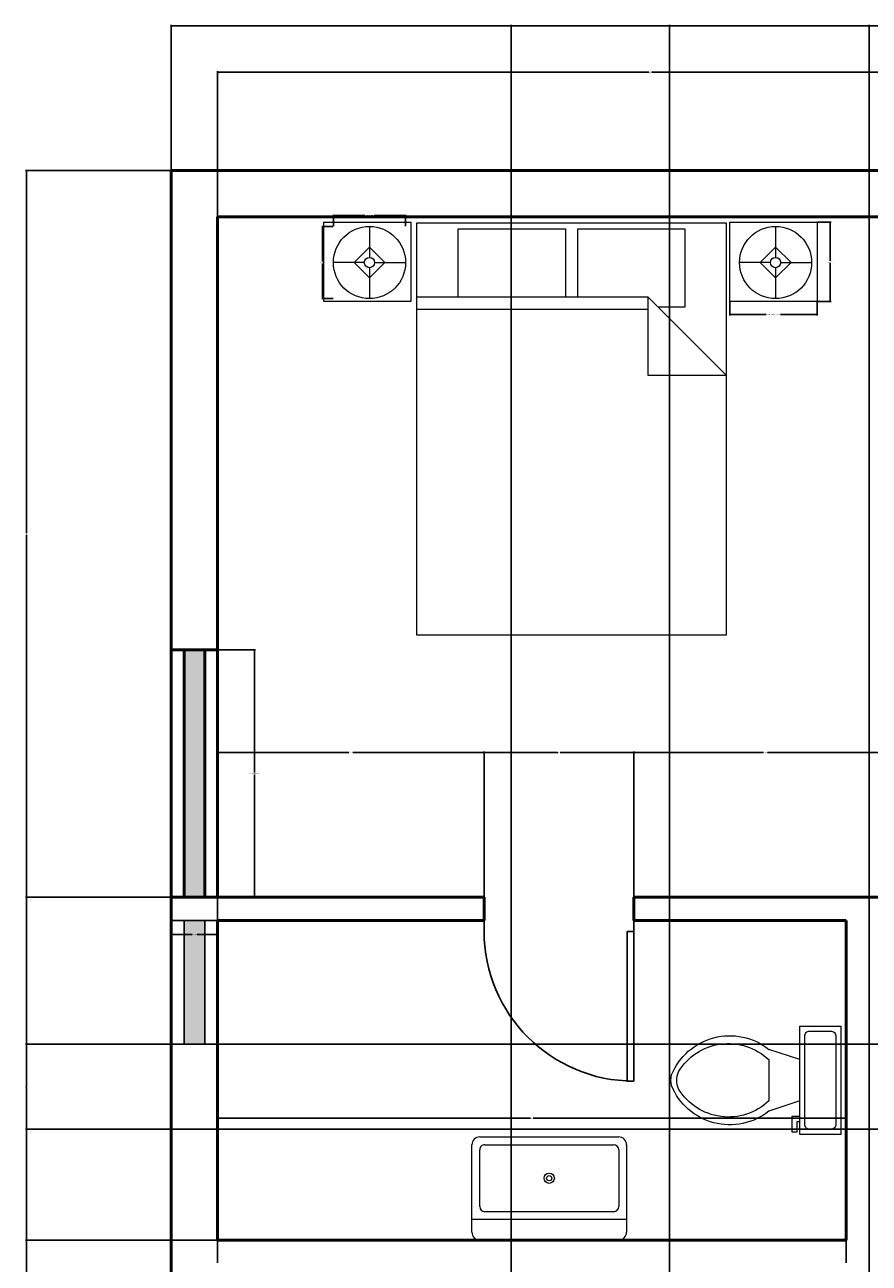
# Model space of a CAD drawing. Units: inches. Extents: x 1974 to 2406, y 1583 to 2170.
# Tile 4 of 6: x 1974 to 2138, y 1930 to 2170. Entities that reach past the tile are written whole.
import ezdxf

# ---------------------------------------------------------------- set-up
doc = ezdxf.new("R2010")
doc.units = ezdxf.units.IN
for name, color, linetype, lineweight in [('A-ANNO-DIMS', 2, 'Continuous', 18), ('A-FLOR-FIXT', 3, 'Continuous', 18), ('A-FURN', 3, 'Continuous', 18), ('A-GLAZ', 4, 'Continuous', 25), ('door', 60, 'Continuous', 25), ('wall', 240, 'Continuous', 50)]:
    doc.layers.add(name, color=color, linetype=linetype, lineweight=lineweight)
doc.styles.get("Standard").update_dxf_attribs({"font": 'arial.ttf'})
doc.dimstyles.get("Standard").update_dxf_attribs({"dimtxt": 0.18, "dimasz": 0.18, "dimexe": 0.18, "dimexo": 0.0625, "dimgap": 0.09, "dimtad": 0, "dimtih": 1, "dimtoh": 1, "dimdec": 4, "dimzin": 0, "dimdsep": 46, "dimtxsty": 'Standard', "dimcen": 0.09, "dimadec": 0, "dimazin": 0, "dimtfac": 1, "dimtdec": 4, "dimtofl": 0, "dimtmove": 0, "dimatfit": 3, "dimfxl": 1, "dimtolj": 1, "dimtzin": 0, "dimarcsym": 0})

# ---------------------------------------------------------------- blocks, each defined once
blk = doc.blocks.new('*U2')
for p, q in [((0, 0), (0, -6)), ((40, 0), (40, -6))]:
    blk.add_line(p, q)
blk.add_lwpolyline([(0, 0), (0, 40), (1.75, 40), (1.75, 0)], close=True)
blk.add_arc((0, 0), 40, 0, 90)
blk = doc.blocks.new('b')
at = {"layer": 'wall'}
h = blk.add_hatch(color=256, dxfattribs=at)
h.dxf.hatch_style = 1
h.paths.add_polyline_path([(6.5, 0), (2.5, 0), (2.5, -48), (6.5, -48)])
for p, q in [((2.5, 0), (2.5, -48)), ((6.5, 0), (6.5, -48))]:
    blk.add_line(p, q, dxfattribs=at)
blk.add_lwpolyline([(0, -48), (9, -48), (9, 0), (0, 0)], close=True, dxfattribs=at)
blk = doc.blocks.new('*U7')
for p, q in [((9.5, -6), (9.5, -2)), ((-10, -8.5), (-8, -8.5)), ((-10, -9.5), (-10, -8.5)), ((-7, -9.5), (-10, -9.5)), ((-8, -8.5), (-8, -8)), ((-7, -8), (-7, -9.5)), ((-4, -8), (-6, -14)), ((4, -8), (6, -14)), ((4, -14), (-4, -14))]:
    blk.add_line(p, q)
blk.add_lwpolyline([(10.5, -8), (10.5, 0), (-10.5, 0), (-10.5, -8)], close=True)
for points in [[(-9.5, -2), (-9.5, -6)], [(8.5, -1), (-8.5, -1)], [(-8.5, -7), (8.5, -7)]]:
    blk.add_lwpolyline(points)
for centre, radius, start, end in [((-8.62, -1.88), 0.884, 81.8699, 188.1301), ((8.62, -1.88), 0.884, 351.8699, 98.1301), ((-8.62, -6.12), 0.884, 171.8699, 278.1301), ((8.62, -6.12), 0.884, 261.8699, 8.1301), ((3.52, -21.58), 12.17, 141.4691, 247.9714), ((4.2, -21.82), 11.33, 136.3677, 238.9468), ((-3.52, -21.58), 12.17, 292.0284, 38.5307), ((-4.2, -21.82), 11.33, 301.053, 43.6321), ((0, -27.88), 4, 245.7318, 294.2682), ((0, -29), 4, 254.8605, 285.1395)]:
    blk.add_arc(centre, radius, start, end)
blk = doc.blocks.new('Sink-single - 30 in top')
blk.add_line((-15, -3.999996), (15, -3.999996))
for points in [[(-13.5, 0), (13.5, 0)], [(-15, -18.499996), (-15, -1.5)], [(15, -1.5), (15, -18.499996)], [(-13.5, -17.499996), (-13.5, -6.499996)], [(-12.5, -5.499996), (12.5, -5.499996)], [(13.5, -6.499996), (13.5, -17.499996)], [(12.5, -18.499996), (-12.5, -18.499996)], [(13.5, -19.999996), (-13.5, -19.999996)]]:
    blk.add_lwpolyline(points)
for radius in [1, 0.5]:
    blk.add_circle((0, -11.999996), radius)
for centre, radius, start, end in [((-13.5, -1.5), 1.5, 90, 180), ((13.5, -1.5), 1.5, 0, 90), ((-12.5, -6.499996), 1, 90, 180), ((12.5, -6.499996), 1, 0, 90), ((-13.5, -18.499996), 1.5, 180, 270), ((-12.5, -17.499996), 1, 180, 270), ((12.5, -17.499996), 1, 270, 0), ((13.5, -18.499996), 1.5, 270, 0)]:
    blk.add_arc(centre, radius, start, end)
blk = doc.blocks.new('Bed - Queen')
for p, q in [((0, -80.00003), (0, 0)), ((0, 0), (59.99999, 0)), ((59.99999, 0), (59.99999, -80.00003)), ((7.99999, -1.2), (28.79998, -1.2)), ((7.99999, -14.4), (7.99999, -1.2)), ((28.79998, -1.2), (28.79998, -14.4)), ((31.19999, -1.2), (51.99999, -1.2)), ((31.19999, -14.4), (31.19999, -1.2)), ((51.99999, -1.2), (51.99999, -16.4)), ((0, -14.4), (44.8, -14.4)), ((59.99999, -29.6), (44.8, -14.4)), ((44.8, -14.4), (44.8, -29.6)), ((44.8, -16.8), (0, -16.8)), ((51.99999, -16.4), (46.79936, -16.4)), ((44.8, -29.6), (59.99999, -29.6)), ((59.99999, -80.00003), (0, -80.00003))]:
    blk.add_line(p, q)
blk = doc.blocks.new('Lamp - Table')
for p, q in [((0, 7), (0, 1)), ((0, 3), (-3, 0)), ((3, 0), (0, 3)), ((-1, 0), (-7, 0)), ((-3, 0), (0, -3)), ((0, -3), (3, 0)), ((1, 0), (7, 0)), ((0, -1), (0, -7))]:
    blk.add_line(p, q)
for radius in [7, 1]:
    blk.add_circle((0, 0), radius)
blk = doc.blocks.new('WINDOW-24IN')
h = blk.add_hatch(color=256)
h.dxf.hatch_style = 1
h.paths.add_polyline_path([(6.5, 24), (2.5, 24), (2.5, 0), (6.5, 0)])
for p, q in [((2.5, 24), (2.5, 0)), ((6.5, 24), (6.5, 0))]:
    blk.add_line(p, q)
blk.add_lwpolyline([(0, 0), (0, 24), (9, 24), (9, 0)], close=True)
blk = doc.blocks.new('TABLE-NIGHTSTAND')
blk.add_lwpolyline([(0, 15.39), (16.93, 15.39), (16.93, 0), (0, 0)], close=True)
blk = doc.blocks.new('*D20')
at = {"layer": 'A-ANNO-DIMS', "color": 0, "lineweight": -2, "transparency": 16777216}
for p, q in [((2033.65, 2131.22), (2033.65, 2133.44)), ((2033.83, 2133.26), (2039.74, 2133.26)), ((2047.47, 2133.26), (2041.55, 2133.26)), ((2047.65, 2131.22), (2047.65, 2133.44))]:
    blk.add_line(p, q, dxfattribs=at)
at = {"layer": 'A-ANNO-DIMS', "color": 0, "transparency": 16777216}
for points in [[(2033.83, 2133.29), (2033.83, 2133.23), (2033.65, 2133.26)], [(2047.47, 2133.29), (2047.47, 2133.23), (2047.65, 2133.26)]]:
    blk.add_solid(points, dxfattribs=at)
at = {"layer": 'Defpoints', "color": 0, "transparency": 16777216}
for p in [(2047.65, 2133.26), (2033.65, 2131.16), (2047.65, 2131.16)]:
    blk.add_point(p, dxfattribs=at)
at = {"layer": 'A-ANNO-DIMS', "color": 0, "transparency": 16777216, "insert": (2040.65, 2133.26), "char_height": 0.18, "attachment_point": 5}
blk.add_mtext('\\A1;LAMP 14 TYP.', dxfattribs=at)
blk = doc.blocks.new('*D21')
at = {"layer": 'A-ANNO-DIMS', "color": 0, "lineweight": -2, "transparency": 16777216}
for p, q in [((2033.58, 2131.16), (2031.37, 2131.16)), ((2031.55, 2130.98), (2031.55, 2124.34)), ((2031.55, 2117.34), (2031.55, 2123.98)), ((2033.58, 2117.16), (2031.37, 2117.16))]:
    blk.add_line(p, q, dxfattribs=at)
at = {"layer": 'A-ANNO-DIMS', "color": 0, "transparency": 16777216}
for points in [[(2031.52, 2130.98), (2031.58, 2130.98), (2031.55, 2131.16)], [(2031.52, 2117.34), (2031.58, 2117.34), (2031.55, 2117.16)]]:
    blk.add_solid(points, dxfattribs=at)
at = {"layer": 'Defpoints', "color": 0, "transparency": 16777216}
for p in [(2031.55, 2131.16), (2033.65, 2131.16), (2033.65, 2117.16)]:
    blk.add_point(p, dxfattribs=at)
at = {"layer": 'A-ANNO-DIMS', "color": 0, "transparency": 16777216, "insert": (2031.55, 2124.16), "char_height": 0.18, "attachment_point": 5}
blk.add_mtext('\\A1;14 TYP.', dxfattribs=at)
blk = doc.blocks.new('*D22')
at = {"layer": 'A-ANNO-DIMS', "color": 0, "lineweight": -2, "transparency": 16777216}
for p, q in [((2011.22, 2048.99), (2018.54, 2048.99)), ((2018.36, 2048.81), (2018.36, 2025.18)), ((2018.36, 2001.17), (2018.36, 2024.81)), ((2011.22, 2000.99), (2018.54, 2000.99))]:
    blk.add_line(p, q, dxfattribs=at)
at = {"layer": 'A-ANNO-DIMS', "color": 0, "transparency": 16777216}
for points in [[(2018.33, 2048.81), (2018.39, 2048.81), (2018.36, 2048.99)], [(2018.33, 2001.17), (2018.39, 2001.17), (2018.36, 2000.99)]]:
    blk.add_solid(points, dxfattribs=at)
at = {"layer": 'Defpoints', "color": 0, "transparency": 16777216}
for p in [(2011.16, 2048.99), (2018.36, 2048.99), (2011.16, 2000.99)]:
    blk.add_point(p, dxfattribs=at)
at = {"layer": 'A-ANNO-DIMS', "color": 0, "transparency": 16777216, "insert": (2018.36, 2024.99), "char_height": 0.18, "attachment_point": 5}
blk.add_mtext('\\A1;WINDOW 48 TYP.', dxfattribs=at)
blk = doc.blocks.new('*D23')
at = {"layer": 'A-ANNO-DIMS', "color": 0, "lineweight": -2, "transparency": 16777216}
for p, q in [((2002.16, 2000.93), (2002.16, 1993.61)), ((2011.16, 2000.93), (2011.16, 1993.61)), ((2002.34, 1993.79), (2006.2, 1993.79)), ((2010.98, 1993.79), (2007.12, 1993.79))]:
    blk.add_line(p, q, dxfattribs=at)
at = {"layer": 'A-ANNO-DIMS', "color": 0, "transparency": 16777216}
for points in [[(2002.34, 1993.82), (2002.34, 1993.76), (2002.16, 1993.79)], [(2010.98, 1993.82), (2010.98, 1993.76), (2011.16, 1993.79)]]:
    blk.add_solid(points, dxfattribs=at)
at = {"layer": 'Defpoints', "color": 0, "transparency": 16777216}
for p in [(2002.16, 2000.99), (2011.16, 2000.99), (2011.16, 1993.79)]:
    blk.add_point(p, dxfattribs=at)
at = {"layer": 'A-ANNO-DIMS', "color": 0, "transparency": 16777216, "insert": (2006.66, 1993.79), "char_height": 0.18, "attachment_point": 5}
blk.add_mtext('\\A1;9 TYP.', dxfattribs=at)
blk = doc.blocks.new('*D32')
at = {"layer": 'A-ANNO-DIMS', "color": 0, "lineweight": -2, "transparency": 16777216}
for p, q in [((2110.59, 2116.54), (2110.59, 2113.89)), ((2127.53, 2116.54), (2127.53, 2113.89)), ((2110.77, 2114.07), (2117.68, 2114.07)), ((2127.35, 2114.07), (2120.44, 2114.07))]:
    blk.add_line(p, q, dxfattribs=at)
at = {"layer": 'A-ANNO-DIMS', "color": 0, "transparency": 16777216}
for points in [[(2110.77, 2114.1), (2110.77, 2114.04), (2110.59, 2114.07)], [(2127.35, 2114.1), (2127.35, 2114.04), (2127.53, 2114.07)]]:
    blk.add_solid(points, dxfattribs=at)
at = {"layer": 'Defpoints', "color": 0, "transparency": 16777216}
for p in [(2110.59, 2116.61), (2127.53, 2116.61), (2127.53, 2114.07)]:
    blk.add_point(p, dxfattribs=at)
at = {"layer": 'A-ANNO-DIMS', "color": 0, "transparency": 16777216, "insert": (2119.06, 2114.07), "char_height": 0.18, "attachment_point": 5}
blk.add_mtext('\\A1;NIGHTSTAND 17 TYP.', dxfattribs=at)
blk = doc.blocks.new('*D33')
at = {"layer": 'A-ANNO-DIMS', "color": 0, "lineweight": -2, "transparency": 16777216}
for p, q in [((2127.59, 2132), (2130.25, 2132)), ((2130.07, 2131.82), (2130.07, 2124.48)), ((2130.07, 2116.79), (2130.07, 2124.12)), ((2127.59, 2116.61), (2130.25, 2116.61))]:
    blk.add_line(p, q, dxfattribs=at)
at = {"layer": 'A-ANNO-DIMS', "color": 0, "transparency": 16777216}
for points in [[(2130.04, 2131.82), (2130.1, 2131.82), (2130.07, 2132)], [(2130.04, 2116.79), (2130.1, 2116.79), (2130.07, 2116.61)]]:
    blk.add_solid(points, dxfattribs=at)
at = {"layer": 'Defpoints', "color": 0, "transparency": 16777216}
for p in [(2127.53, 2132), (2130.07, 2132), (2127.53, 2116.61)]:
    blk.add_point(p, dxfattribs=at)
at = {"layer": 'A-ANNO-DIMS', "color": 0, "transparency": 16777216, "insert": (2130.07, 2124.3), "char_height": 0.18, "attachment_point": 5}
blk.add_mtext('\\A1;15 TYP.', dxfattribs=at)
blk = doc.blocks.new('*D48')
at = {"layer": 'A-ANNO-DIMS', "color": 0, "lineweight": -2, "transparency": 16777216}
for p, q in [((2002.16, 2142.05), (2002.16, 2170.29)), ((2002.34, 2170.11), (2189.51, 2170.11)), ((2377.48, 2170.11), (2190.3, 2170.11)), ((2377.66, 2142.05), (2377.66, 2170.29))]:
    blk.add_line(p, q, dxfattribs=at)
at = {"layer": 'A-ANNO-DIMS', "color": 0, "transparency": 16777216}
for points in [[(2002.34, 2170.14), (2002.34, 2170.08), (2002.16, 2170.11)], [(2377.48, 2170.14), (2377.48, 2170.08), (2377.66, 2170.11)]]:
    blk.add_solid(points, dxfattribs=at)
at = {"layer": 'Defpoints', "color": 0, "transparency": 16777216}
for p in [(2377.66, 2170.11), (2002.16, 2141.99), (2377.66, 2141.99)]:
    blk.add_point(p, dxfattribs=at)
at = {"layer": 'A-ANNO-DIMS', "color": 0, "transparency": 16777216, "insert": (2189.91, 2170.11), "char_height": 0.18, "attachment_point": 5}
blk.add_mtext('\\A1;375.5', dxfattribs=at)
blk = doc.blocks.new('*D50')
at = {"layer": 'A-ANNO-DIMS', "color": 0, "lineweight": -2, "transparency": 16777216}
for p, q in [((2011.16, 2133.05), (2011.16, 2161.29)), ((2011.34, 2161.11), (2094.88, 2161.11)), ((2178.98, 2161.11), (2095.44, 2161.11)), ((2179.16, 2133.05), (2179.16, 2161.29))]:
    blk.add_line(p, q, dxfattribs=at)
at = {"layer": 'A-ANNO-DIMS', "color": 0, "transparency": 16777216}
for points in [[(2011.34, 2161.14), (2011.34, 2161.08), (2011.16, 2161.11)], [(2178.98, 2161.14), (2178.98, 2161.08), (2179.16, 2161.11)]]:
    blk.add_solid(points, dxfattribs=at)
at = {"layer": 'Defpoints', "color": 0, "transparency": 16777216}
for p in [(2179.16, 2161.11), (2011.16, 2132.99), (2179.16, 2132.99)]:
    blk.add_point(p, dxfattribs=at)
at = {"layer": 'A-ANNO-DIMS', "color": 0, "transparency": 16777216, "insert": (2095.16, 2161.11), "char_height": 0.18, "attachment_point": 5}
blk.add_mtext('\\A1;168', dxfattribs=at)
blk = doc.blocks.new('*D54')
at = {"layer": 'A-ANNO-DIMS', "color": 0, "lineweight": -2, "transparency": 16777216}
for p, q in [((2002.1, 2141.99), (1973.86, 2141.99)), ((1974.04, 2141.81), (1974.04, 2071.67)), ((1974.04, 2001.17), (1974.04, 2071.31)), ((2011.1, 2000.99), (1973.86, 2000.99))]:
    blk.add_line(p, q, dxfattribs=at)
at = {"layer": 'A-ANNO-DIMS', "color": 0, "transparency": 16777216}
for points in [[(1974.01, 2141.81), (1974.07, 2141.81), (1974.04, 2141.99)], [(1974.01, 2001.17), (1974.07, 2001.17), (1974.04, 2000.99)]]:
    blk.add_solid(points, dxfattribs=at)
at = {"layer": 'Defpoints', "color": 0, "transparency": 16777216}
for p in [(2002.16, 2141.99), (1974.04, 2000.99), (2011.16, 2000.99)]:
    blk.add_point(p, dxfattribs=at)
at = {"layer": 'A-ANNO-DIMS', "color": 0, "transparency": 16777216, "insert": (1974.04, 2071.49), "char_height": 0.18, "attachment_point": 5}
blk.add_mtext('\\A1;141', dxfattribs=at)
blk = doc.blocks.new('*D55')
at = {"layer": 'A-ANNO-DIMS', "color": 0, "lineweight": -2, "transparency": 16777216}
for p, q in [((2011.1, 2000.99), (1973.86, 2000.99)), ((1974.04, 2000.81), (1974.04, 1967.92)), ((1974.04, 1934.67), (1974.04, 1967.56)), ((2011.1, 1934.49), (1973.86, 1934.49))]:
    blk.add_line(p, q, dxfattribs=at)
at = {"layer": 'A-ANNO-DIMS', "color": 0, "transparency": 16777216}
for points in [[(1974.01, 2000.81), (1974.07, 2000.81), (1974.04, 2000.99)], [(1974.01, 1934.67), (1974.07, 1934.67), (1974.04, 1934.49)]]:
    blk.add_solid(points, dxfattribs=at)
at = {"layer": 'Defpoints', "color": 0, "transparency": 16777216}
for p in [(2011.16, 2000.99), (1974.04, 1934.49), (2011.16, 1934.49)]:
    blk.add_point(p, dxfattribs=at)
at = {"layer": 'A-ANNO-DIMS', "color": 0, "transparency": 16777216, "insert": (1974.04, 1967.74), "char_height": 0.18, "attachment_point": 5}
blk.add_mtext('\\A1;66.5', dxfattribs=at)
blk = doc.blocks.new('*D56')
at = {"layer": 'A-ANNO-DIMS', "color": 0, "lineweight": -2, "transparency": 16777216}
for p, q in [((2011.1, 1934.49), (1973.86, 1934.49)), ((1974.04, 1934.31), (1974.04, 1871.92)), ((1974.04, 1809.17), (1974.04, 1871.56)), ((2011.1, 1808.99), (1973.86, 1808.99))]:
    blk.add_line(p, q, dxfattribs=at)
at = {"layer": 'A-ANNO-DIMS', "color": 0, "transparency": 16777216}
for points in [[(1974.01, 1934.31), (1974.07, 1934.31), (1974.04, 1934.49)], [(1974.01, 1809.17), (1974.07, 1809.17), (1974.04, 1808.99)]]:
    blk.add_solid(points, dxfattribs=at)
at = {"layer": 'Defpoints', "color": 0, "transparency": 16777216}
for p in [(2011.16, 1934.49), (1974.04, 1808.99), (2011.16, 1808.99)]:
    blk.add_point(p, dxfattribs=at)
at = {"layer": 'A-ANNO-DIMS', "color": 0, "transparency": 16777216, "insert": (1974.04, 1871.74), "char_height": 0.18, "attachment_point": 5}
blk.add_mtext('\\A1;125.5', dxfattribs=at)
blk = doc.blocks.new('*D65')
at = {"layer": 'A-ANNO-DIMS', "color": 0, "lineweight": -2, "transparency": 16777216}
for p, q in [((2011.16, 1930.05), (2011.16, 1958.29)), ((2011.34, 1958.11), (2071.88, 1958.11)), ((2132.98, 1958.11), (2072.44, 1958.11)), ((2133.16, 1930.05), (2133.16, 1958.29))]:
    blk.add_line(p, q, dxfattribs=at)
at = {"layer": 'A-ANNO-DIMS', "color": 0, "transparency": 16777216}
for points in [[(2011.34, 1958.14), (2011.34, 1958.08), (2011.16, 1958.11)], [(2132.98, 1958.14), (2132.98, 1958.08), (2133.16, 1958.11)]]:
    blk.add_solid(points, dxfattribs=at)
at = {"layer": 'Defpoints', "color": 0, "transparency": 16777216}
for p in [(2133.16, 1958.11), (2011.16, 1929.99), (2133.16, 1929.99)]:
    blk.add_point(p, dxfattribs=at)
at = {"layer": 'A-ANNO-DIMS', "color": 0, "transparency": 16777216, "insert": (2072.16, 1958.11), "char_height": 0.18, "attachment_point": 5}
blk.add_mtext('\\A1;122', dxfattribs=at)
blk = doc.blocks.new('*D66')
at = {"layer": 'A-ANNO-DIMS', "color": 0, "lineweight": -2, "transparency": 16777216}
for p, q in [((2062.94, 2001.05), (2062.94, 2029.29)), ((2063.12, 2029.11), (2077.22, 2029.11)), ((2091.76, 2029.11), (2077.66, 2029.11)), ((2091.94, 2001.05), (2091.94, 2029.29))]:
    blk.add_line(p, q, dxfattribs=at)
at = {"layer": 'A-ANNO-DIMS', "color": 0, "transparency": 16777216}
for points in [[(2063.12, 2029.14), (2063.12, 2029.08), (2062.94, 2029.11)], [(2091.76, 2029.14), (2091.76, 2029.08), (2091.94, 2029.11)]]:
    blk.add_solid(points, dxfattribs=at)
at = {"layer": 'Defpoints', "color": 0, "transparency": 16777216}
for p in [(2091.94, 2029.11), (2062.94, 2000.99), (2091.94, 2000.99)]:
    blk.add_point(p, dxfattribs=at)
at = {"layer": 'A-ANNO-DIMS', "color": 0, "transparency": 16777216, "insert": (2077.44, 2029.11), "char_height": 0.18, "attachment_point": 5}
blk.add_mtext('\\A1;29', dxfattribs=at)
blk = doc.blocks.new('*D67')
at = {"layer": 'A-ANNO-DIMS', "color": 0, "lineweight": -2, "transparency": 16777216}
for p, q in [((2011.16, 2001.05), (2011.16, 2029.29)), ((2011.34, 2029.11), (2036.66, 2029.11)), ((2062.76, 2029.11), (2037.44, 2029.11)), ((2062.94, 2001.05), (2062.94, 2029.29))]:
    blk.add_line(p, q, dxfattribs=at)
at = {"layer": 'A-ANNO-DIMS', "color": 0, "transparency": 16777216}
for points in [[(2011.34, 2029.14), (2011.34, 2029.08), (2011.16, 2029.11)], [(2062.76, 2029.14), (2062.76, 2029.08), (2062.94, 2029.11)]]:
    blk.add_solid(points, dxfattribs=at)
at = {"layer": 'Defpoints', "color": 0, "transparency": 16777216}
for p in [(2062.94, 2029.11), (2011.16, 2000.99), (2062.94, 2000.99)]:
    blk.add_point(p, dxfattribs=at)
at = {"layer": 'A-ANNO-DIMS', "color": 0, "transparency": 16777216, "insert": (2037.05, 2029.11), "char_height": 0.18, "attachment_point": 5}
blk.add_mtext('\\A1;51.78', dxfattribs=at)
blk = doc.blocks.new('*D69')
at = {"layer": 'A-ANNO-DIMS', "color": 0, "lineweight": -2, "transparency": 16777216}
for p, q in [((2091.94, 2001.05), (2091.94, 2029.29)), ((2092.12, 2029.11), (2117.16, 2029.11)), ((2142.98, 2029.11), (2117.94, 2029.11)), ((2143.16, 2001.05), (2143.16, 2029.29))]:
    blk.add_line(p, q, dxfattribs=at)
at = {"layer": 'A-ANNO-DIMS', "color": 0, "transparency": 16777216}
for points in [[(2092.12, 2029.14), (2092.12, 2029.08), (2091.94, 2029.11)], [(2142.98, 2029.14), (2142.98, 2029.08), (2143.16, 2029.11)]]:
    blk.add_solid(points, dxfattribs=at)
at = {"layer": 'Defpoints', "color": 0, "transparency": 16777216}
for p in [(2143.16, 2029.11), (2091.94, 2000.99), (2143.16, 2000.99)]:
    blk.add_point(p, dxfattribs=at)
at = {"layer": 'A-ANNO-DIMS', "color": 0, "transparency": 16777216, "insert": (2117.55, 2029.11), "char_height": 0.18, "attachment_point": 5}
blk.add_mtext('\\A1;51.22', dxfattribs=at)
blk = doc.blocks.new('*D73')
at = {"layer": 'A-ANNO-DIMS', "color": 0, "lineweight": -2, "transparency": 16777216}
for p, q in [((2258.6, 1972.49), (1973.86, 1972.49)), ((1974.04, 1972.31), (1974.04, 1941.67)), ((1974.04, 1910.67), (1974.04, 1941.31)), ((2254.1, 1910.49), (1973.86, 1910.49))]:
    blk.add_line(p, q, dxfattribs=at)
at = {"layer": 'A-ANNO-DIMS', "color": 0, "transparency": 16777216}
for points in [[(1974.01, 1972.31), (1974.07, 1972.31), (1974.04, 1972.49)], [(1974.01, 1910.67), (1974.07, 1910.67), (1974.04, 1910.49)]]:
    blk.add_solid(points, dxfattribs=at)
at = {"layer": 'Defpoints', "color": 0, "transparency": 16777216}
for p in [(2258.66, 1972.49), (1974.04, 1910.49), (2254.16, 1910.49)]:
    blk.add_point(p, dxfattribs=at)
at = {"layer": 'A-ANNO-DIMS', "color": 0, "transparency": 16777216, "insert": (1974.04, 1941.49), "char_height": 0.18, "attachment_point": 5}
blk.add_mtext('\\A1;62', dxfattribs=at)
blk = doc.blocks.new('*D81')
at = {"layer": 'A-ANNO-DIMS', "color": 0, "lineweight": -2, "transparency": 16777216}
for p, q in [((2258.6, 1972.49), (1973.86, 1972.49)), ((1974.04, 1972.31), (1974.04, 1964.42)), ((1974.04, 1956.17), (1974.04, 1964.06)), ((2258.6, 1955.99), (1973.86, 1955.99))]:
    blk.add_line(p, q, dxfattribs=at)
at = {"layer": 'A-ANNO-DIMS', "color": 0, "transparency": 16777216}
for points in [[(1974.01, 1972.31), (1974.07, 1972.31), (1974.04, 1972.49)], [(1974.01, 1956.17), (1974.07, 1956.17), (1974.04, 1955.99)]]:
    blk.add_solid(points, dxfattribs=at)
at = {"layer": 'Defpoints', "color": 0, "transparency": 16777216}
for p in [(1974.04, 1972.49), (2258.66, 1972.49), (2258.66, 1955.99)]:
    blk.add_point(p, dxfattribs=at)
at = {"layer": 'A-ANNO-DIMS', "color": 0, "transparency": 16777216, "insert": (1974.04, 1964.24), "char_height": 0.18, "attachment_point": 5}
blk.add_mtext('\\A1;16.5', dxfattribs=at)
blk = doc.blocks.new('*D93')
at = {"layer": 'A-ANNO-DIMS', "color": 0, "lineweight": -2, "transparency": 16777216}
for p, q in [((2068.16, 1728.05), (2068.16, 2170.29)), ((2068.34, 2170.11), (2083.07, 2170.11)), ((2098.72, 2170.11), (2083.99, 2170.11)), ((2098.9, 1721.56), (2098.9, 2170.29))]:
    blk.add_line(p, q, dxfattribs=at)
at = {"layer": 'A-ANNO-DIMS', "color": 0, "transparency": 16777216}
for points in [[(2068.34, 2170.14), (2068.34, 2170.08), (2068.16, 2170.11)], [(2098.72, 2170.14), (2098.72, 2170.08), (2098.9, 2170.11)]]:
    blk.add_solid(points, dxfattribs=at)
at = {"layer": 'Defpoints', "color": 0, "transparency": 16777216}
for p in [(2098.9, 2170.11), (2068.16, 1727.99), (2098.9, 1721.49)]:
    blk.add_point(p, dxfattribs=at)
at = {"layer": 'A-ANNO-DIMS', "color": 0, "transparency": 16777216, "insert": (2083.53, 2170.11), "char_height": 0.18, "attachment_point": 5}
blk.add_mtext('\\A1;30.746', dxfattribs=at)
blk = doc.blocks.new('*D94')
at = {"layer": 'A-ANNO-DIMS', "color": 0, "lineweight": -2, "transparency": 16777216}
for p, q in [((2068.16, 1800.05), (2068.16, 2170.29)), ((2068.34, 2170.11), (2102.58, 2170.11)), ((2137.48, 2170.11), (2103.23, 2170.11)), ((2137.66, 1800.05), (2137.66, 2170.29))]:
    blk.add_line(p, q, dxfattribs=at)
at = {"layer": 'A-ANNO-DIMS', "color": 0, "transparency": 16777216}
for points in [[(2068.34, 2170.14), (2068.34, 2170.08), (2068.16, 2170.11)], [(2137.48, 2170.14), (2137.48, 2170.08), (2137.66, 2170.11)]]:
    blk.add_solid(points, dxfattribs=at)
at = {"layer": 'Defpoints', "color": 0, "transparency": 16777216}
for p in [(2137.66, 2170.11), (2068.16, 1799.99), (2137.66, 1799.99)]:
    blk.add_point(p, dxfattribs=at)
at = {"layer": 'A-ANNO-DIMS', "color": 0, "transparency": 16777216, "insert": (2102.91, 2170.11), "char_height": 0.18, "attachment_point": 5}
blk.add_mtext('\\A1;69.5', dxfattribs=at)

msp = doc.modelspace()

# ---------------------------------------------------------------- linework, layer by layer
at = {"layer": 'wall'}
for p, q in [((2002.1581, 2141.9921), (2002.1581, 1694.9921)), ((2002.1581, 2141.9921), (2206.8193, 2141.9921)), ((2011.1581, 2132.9921), (2011.1581, 2000.9921)), ((2011.1581, 2132.9921), (2179.1581, 2132.9921)), ((2011.1581, 2000.9921), (2062.9418, 2000.9921)), ((2062.9418, 2000.9921), (2062.9418, 1996.4921)), ((2091.9418, 2000.9921), (2091.9418, 1996.4921)), ((2091.9418, 2000.9921), (2143.1581, 2000.9921)), ((2011.1581, 1996.4921), (2062.9418, 1996.4921)), ((2011.1581, 1996.4921), (2011.1581, 1934.4921)), ((2091.9418, 1996.4921), (2133.1581, 1996.4921)), ((2133.1581, 1996.4921), (2133.1581, 1934.4921)), ((2011.1581, 1934.4921), (2133.1581, 1934.4921))]:
    msp.add_line(p, q, dxfattribs=at)

# ---------------------------------------------------------------- block references
at = {"layer": 'A-FLOR-FIXT', "xscale": -1, "rotation": 270}
msp.add_blockref('*U7', (2132.1581, 1965.4921), dxfattribs=at)
at = {"layer": 'A-FLOR-FIXT', "rotation": 180}
msp.add_blockref('Sink-single - 30 in top', (2075.5375, 1934.4921), dxfattribs=at)
at = {"layer": 'A-FURN'}
for name, p in [('TABLE-NIGHTSTAND', (2031.7641, 2116.607)), ('Bed - Queen', (2049.8724, 2131.874)), ('TABLE-NIGHTSTAND', (2110.595, 2116.607)), ('Lamp - Table', (2040.6452, 2124.1555)), ('Lamp - Table', (2119.476, 2124.1555))]:
    msp.add_blockref(name, p, dxfattribs=at)
at = {"layer": 'A-GLAZ'}
for name, p in [('b', (2002.1581, 2048.9921)), ('WINDOW-24IN', (2002.158, 1972.492))]:
    msp.add_blockref(name, p, dxfattribs=at)
at = {"layer": 'door', "xscale": 0.7261744561551607, "yscale": 0.7261744561551607, "zscale": 0.7261744561551607, "rotation": 179.9999999999992}
msp.add_blockref('*U2', (2091.9418, 1994.3851), dxfattribs=at)

# ---------------------------------------------------------------- dimensions: what is measured, and where the dimension line sits
at = {"layer": 'A-ANNO-DIMS'}
for base, p1, p2, override, picture, middle in [((2377.6581, 2170.1096), (2002.1581, 2141.9921), (2377.6581, 2141.9921), {"dimdec": 1, "dimlfac": 1, "dimrnd": 0, "dimzin": 0, "dimdsep": 46, "dimlunit": 2}, '*D48', (2189.9081, 2170.1096)), ((2098.9039, 2170.1096), (2068.1581, 1727.9921), (2098.9039, 1721.4943), {"dimdec": 3, "dimlfac": 1, "dimrnd": 0, "dimzin": 0, "dimdsep": 46, "dimlunit": 2}, '*D93', (2083.531, 2170.1096)), ((2137.6581, 2170.1096), (2068.1581, 1799.9921), (2137.6581, 1799.9921), {"dimdec": 1, "dimlfac": 1, "dimrnd": 0, "dimzin": 0, "dimdsep": 46, "dimlunit": 2}, '*D94', (2102.9081, 2170.1096)), ((2179.1581, 2161.1096), (2011.1581, 2132.9921), (2179.1581, 2132.9921), {"dimdec": 0, "dimlfac": 1, "dimrnd": 0, "dimzin": 0, "dimdsep": 46, "dimlunit": 2}, '*D50', (2095.1581, 2161.1096)), ((2062.9418, 2029.1096), (2011.1581, 2000.9921), (2062.9418, 2000.9921), {"dimdec": 2, "dimlfac": 1, "dimrnd": 0, "dimzin": 0, "dimdsep": 46, "dimlunit": 2}, '*D67', (2037.0499, 2029.1096)), ((2091.9418, 2029.1096), (2062.9418, 2000.9921), (2091.9418, 2000.9921), {"dimdec": 0, "dimlfac": 1, "dimrnd": 0, "dimzin": 0, "dimdsep": 46, "dimlunit": 2}, '*D66', (2077.4418, 2029.1096)), ((2143.1581, 2029.1096), (2091.9418, 2000.9921), (2143.1581, 2000.9921), {"dimdec": 2, "dimlfac": 1, "dimrnd": 0, "dimzin": 0, "dimdsep": 46, "dimlunit": 2}, '*D69', (2117.5499, 2029.1096)), ((2133.1581, 1958.1096), (2011.1581, 1929.9921), (2133.1581, 1929.9921), {"dimdec": 0, "dimlfac": 1, "dimrnd": 0, "dimzin": 0, "dimdsep": 46, "dimlunit": 2}, '*D65', (2072.1581, 1958.1096))]:
    dim = msp.add_linear_dim(base=base, p1=p1, p2=p2, dimstyle='Standard', override=override, dxfattribs=at)
    dim.commit()
    dim.dimension.update_dxf_attribs({"geometry": picture, "text_midpoint": middle})
for base, p1, p2, override, picture, middle in [((1974.0406, 2000.9921), (2002.1581, 2141.9921), (2011.1581, 2000.9921), {"dimdec": 0, "dimlfac": 1, "dimrnd": 0, "dimzin": 0, "dimdsep": 46, "dimlunit": 2}, '*D54', (1974.0406, 2071.4921)), ((1974.0406, 1934.4921), (2011.1581, 2000.9921), (2011.1581, 1934.4921), {"dimdec": 1, "dimlfac": 1, "dimrnd": 0, "dimzin": 0, "dimdsep": 46, "dimlunit": 2}, '*D55', (1974.0406, 1967.7421)), ((1974.0406, 1972.4921), (2258.6581, 1955.9921), (2258.6581, 1972.4921), {"dimdec": 1, "dimlfac": 1, "dimrnd": 0, "dimzin": 0, "dimdsep": 46, "dimlunit": 2}, '*D81', (1974.0406, 1964.2421)), ((1974.0406, 1910.4921), (2258.6581, 1972.4921), (2254.1581, 1910.4921), {"dimdec": 0, "dimlfac": 1, "dimrnd": 0, "dimzin": 0, "dimdsep": 46, "dimlunit": 2}, '*D73', (1974.0406, 1941.4921)), ((1974.0406, 1808.9921), (2011.1581, 1934.4921), (2011.1581, 1808.9921), {"dimdec": 1, "dimlfac": 1, "dimrnd": 0, "dimzin": 0, "dimdsep": 46, "dimlunit": 2}, '*D56', (1974.0406, 1871.7421))]:
    dim = msp.add_linear_dim(base=base, p1=p1, p2=p2, angle=90, dimstyle='Standard', override=override, dxfattribs=at)
    dim.commit()
    dim.dimension.update_dxf_attribs({"geometry": picture, "text_midpoint": middle})
for base, p1, p2, text, picture, middle in [((2047.6452, 2133.2555), (2033.6452, 2131.1555), (2047.6452, 2131.1555), 'LAMP <> TYP.', '*D20', (2040.6452, 2133.2555)), ((2127.5267, 2114.0672), (2110.5947, 2116.607), (2127.5267, 2116.607), 'NIGHTSTAND <> TYP.', '*D32', (2119.0607, 2114.0672)), ((2011.1581, 1993.7921), (2002.1581, 2000.9921), (2011.1581, 2000.9921), '<> TYP.', '*D23', (2006.6581, 1993.7921))]:
    dim = msp.add_linear_dim(base=base, p1=p1, p2=p2, text=text, dimstyle='Standard', override={"dimdec": 0, "dimlfac": 1, "dimrnd": 0, "dimzin": 0, "dimdsep": 46, "dimlunit": 2}, dxfattribs=at)
    dim.commit()
    dim.dimension.update_dxf_attribs({"geometry": picture, "text_midpoint": middle})
for base, p1, p2, text, picture, middle in [((2130.0665, 2131.9976), (2127.5267, 2116.607), (2127.5267, 2131.9976), '<> TYP.', '*D33', (2130.0665, 2124.3023)), ((2031.5452, 2131.1555), (2033.6452, 2117.1555), (2033.6452, 2131.1555), '<> TYP.', '*D21', (2031.5452, 2124.1555)), ((2018.3581, 2048.9921), (2011.1581, 2000.9921), (2011.1581, 2048.9921), 'WINDOW <> TYP.', '*D22', (2018.3581, 2024.9921))]:
    dim = msp.add_linear_dim(base=base, p1=p1, p2=p2, angle=90, text=text, dimstyle='Standard', override={"dimdec": 0, "dimlfac": 1, "dimrnd": 0, "dimzin": 0, "dimdsep": 46, "dimlunit": 2}, dxfattribs=at)
    dim.commit()
    dim.dimension.update_dxf_attribs({"geometry": picture, "text_midpoint": middle})

doc.saveas('drawing.dxf')
